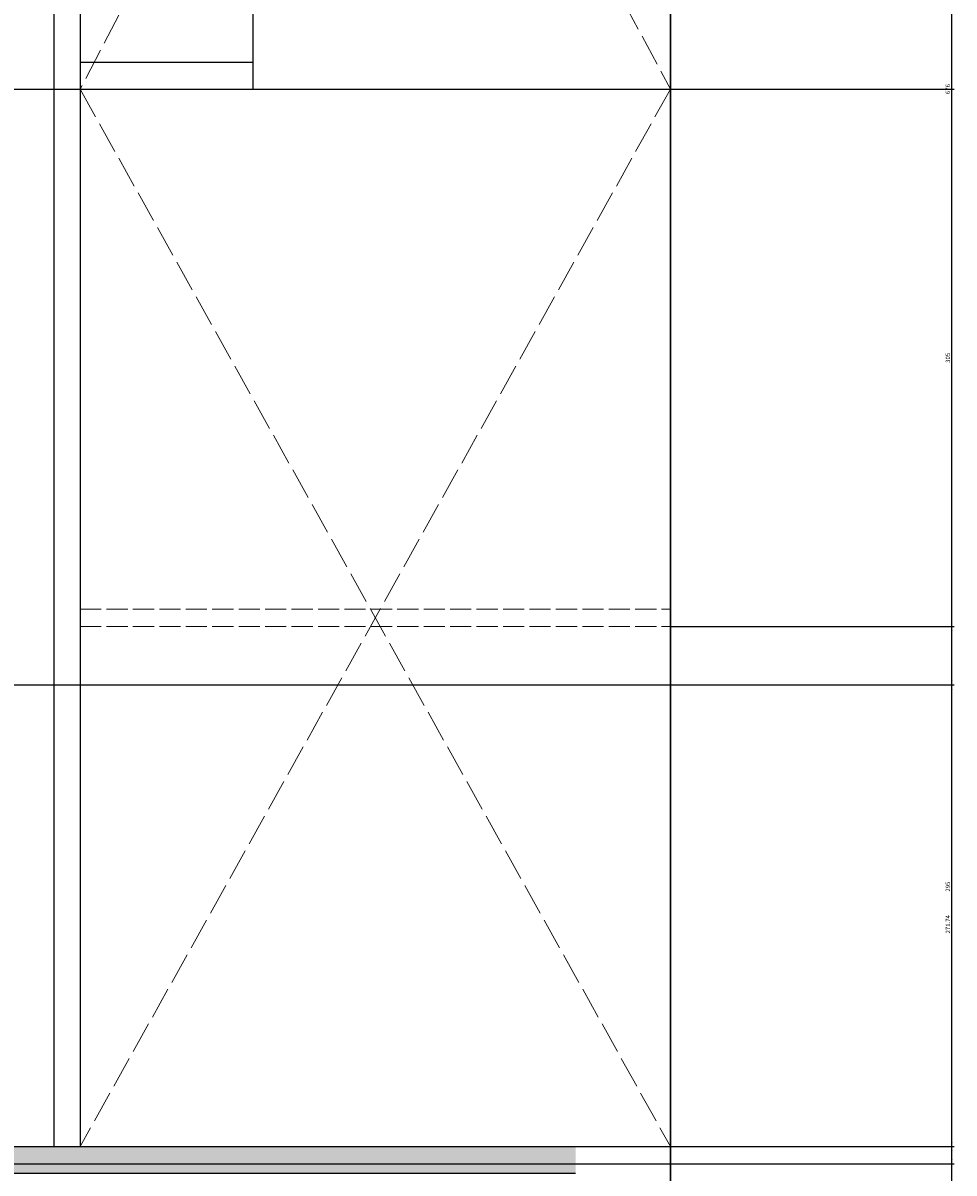
# Model space of a CAD drawing. Units: millimetres. Extents: x 2332 to 5836, y -853 to 2199.
# Tile 15 of 16: x 5308 to 5836, y 753 to 1405. Entities that reach past the tile are written whole.
import ezdxf

# ---------------------------------------------------------------- set-up
doc = ezdxf.new("R2010")
doc.units = ezdxf.units.MM
doc.linetypes.add('ACAD_ISO02W100', pattern=[15, 12, -3])
doc.layers.get('0').update_dxf_attribs({"color": 8})
for name, color, linetype, lineweight in [('A-ANNO-DIMS', 2, 'Continuous', 18), ('A-CSWK-HIDN', 8, 'ACAD_ISO02W100', 13), ('A-CSWK-PATT', 40, 'Continuous', 13), ('A-WALL', 8, 'Continuous', 30), ('SHELF', 40, 'Continuous', 25)]:
    doc.layers.add(name, color=color, linetype=linetype, lineweight=lineweight)
doc.styles.get("Standard").update_dxf_attribs({"font": 'arial.ttf'})
doc.dimstyles.new('ISO-25', dxfattribs={"dimtxt": 2.5, "dimasz": 2.5, "dimexe": 1.25, "dimexo": 0.625, "dimtad": 1, "dimtxsty": 'Standard', "dimcen": 2.5, "dimadec": 0, "dimazin": 0, "dimtfac": 1, "dimtmove": 0, "dimatfit": 3, "dimfxl": 1, "dimarcsym": 0})

# ---------------------------------------------------------------- blocks, each defined once
blk = doc.blocks.new('CAB-END-STILE')
for p, q in [((0, 1240), (0, 600)), ((98.09, 1240), (98.09, 0)), ((113.09, 1240), (113.09, 0)), ((0, 615), (98.09, 615))]:
    blk.add_line(p, q)
blk = doc.blocks.new('*D18')
at = {"layer": 'A-ANNO-DIMS', "color": 0, "lineweight": -2, "transparency": 16777216}
for p, q in [((5675.66, 767.8), (5835.94, 767.8)), ((5834.69, -689.7), (5834.69, 765.3)), ((5675.66, -692.2), (5835.94, -692.2))]:
    blk.add_line(p, q, dxfattribs=at)
at = {"layer": 'A-ANNO-DIMS', "color": 0, "transparency": 16777216}
for points in [[(5834.27, 765.3), (5835.11, 765.3), (5834.69, 767.8)], [(5834.27, -689.7), (5835.11, -689.7), (5834.69, -692.2)]]:
    blk.add_solid(points, dxfattribs=at)
at = {"layer": 'Defpoints', "color": 0, "transparency": 16777216}
for p in [(5675.04, 767.8), (5834.69, 767.8), (5675.04, -692.2)]:
    blk.add_point(p, dxfattribs=at)
at = {"layer": 'A-ANNO-DIMS', "color": 0, "transparency": 16777216, "insert": (5832.79, 37.8), "char_height": 2.5, "attachment_point": 5, "rotation": 90}
blk.add_mtext('1460', dxfattribs=at)
blk = doc.blocks.new('*D19')
at = {"layer": 'A-ANNO-DIMS', "color": 0, "lineweight": -2, "transparency": 16777216}
for p, q in [((5675.66, 1062.8), (5835.94, 1062.8)), ((5834.69, 770.3), (5834.69, 1060.3)), ((5675.66, 767.8), (5835.94, 767.8))]:
    blk.add_line(p, q, dxfattribs=at)
at = {"layer": 'A-ANNO-DIMS', "color": 0, "transparency": 16777216}
for points in [[(5834.27, 1060.3), (5835.11, 1060.3), (5834.69, 1062.8)], [(5834.27, 770.3), (5835.11, 770.3), (5834.69, 767.8)]]:
    blk.add_solid(points, dxfattribs=at)
at = {"layer": 'Defpoints', "color": 0, "transparency": 16777216}
for p in [(5675.04, 1062.8), (5834.69, 1062.8), (5675.04, 767.8)]:
    blk.add_point(p, dxfattribs=at)
at = {"layer": 'A-ANNO-DIMS', "color": 0, "transparency": 16777216, "insert": (5832.79, 915.3), "char_height": 2.5, "attachment_point": 5, "rotation": 90}
blk.add_mtext('295', dxfattribs=at)
blk = doc.blocks.new('*D20')
at = {"layer": 'A-ANNO-DIMS', "color": 0, "lineweight": -2, "transparency": 16777216}
for p, q in [((5675.66, 1367.8), (5835.94, 1367.8)), ((5834.69, 1065.3), (5834.69, 1365.3)), ((5675.66, 1062.8), (5835.94, 1062.8))]:
    blk.add_line(p, q, dxfattribs=at)
at = {"layer": 'A-ANNO-DIMS', "color": 0, "transparency": 16777216}
for points in [[(5834.27, 1365.3), (5835.11, 1365.3), (5834.69, 1367.8)], [(5834.27, 1065.3), (5835.11, 1065.3), (5834.69, 1062.8)]]:
    blk.add_solid(points, dxfattribs=at)
at = {"layer": 'Defpoints', "color": 0, "transparency": 16777216}
for p in [(5675.04, 1367.8), (5834.69, 1367.8), (5675.04, 1062.8)]:
    blk.add_point(p, dxfattribs=at)
at = {"layer": 'A-ANNO-DIMS', "color": 0, "transparency": 16777216, "insert": (5832.79, 1215.3), "char_height": 2.5, "attachment_point": 5, "rotation": 90}
blk.add_mtext('305', dxfattribs=at)
blk = doc.blocks.new('*D25')
at = {"layer": 'A-ANNO-DIMS', "color": 0, "lineweight": -2, "transparency": 16777216}
for p, q in [((4341.52, 1705.81), (5835.94, 1705.81)), ((5834.69, 1032.3), (5834.69, 1703.31)), ((4341.52, 1029.8), (5835.94, 1029.8))]:
    blk.add_line(p, q, dxfattribs=at)
at = {"layer": 'A-ANNO-DIMS', "color": 0, "transparency": 16777216}
for points in [[(5834.27, 1703.31), (5835.11, 1703.31), (5834.69, 1705.81)], [(5834.27, 1032.3), (5835.11, 1032.3), (5834.69, 1029.8)]]:
    blk.add_solid(points, dxfattribs=at)
at = {"layer": 'Defpoints', "color": 0, "transparency": 16777216}
for p in [(4340.89, 1705.81), (5834.69, 1705.81), (4340.89, 1029.8)]:
    blk.add_point(p, dxfattribs=at)
at = {"layer": 'A-ANNO-DIMS', "color": 0, "transparency": 16777216, "insert": (5832.79, 1367.8), "char_height": 2.5, "attachment_point": 5, "rotation": 90}
blk.add_mtext('676', dxfattribs=at)
blk = doc.blocks.new('*D26')
at = {"layer": 'A-ANNO-DIMS', "color": 0, "lineweight": -2, "transparency": 16777216}
for p, q in [((4774.24, 1029.8), (5835.94, 1029.8)), ((5834.69, 760.56), (5834.69, 1027.3)), ((4741.16, 758.06), (5835.94, 758.06))]:
    blk.add_line(p, q, dxfattribs=at)
at = {"layer": 'A-ANNO-DIMS', "color": 0, "transparency": 16777216}
for points in [[(5834.27, 1027.3), (5835.11, 1027.3), (5834.69, 1029.8)], [(5834.27, 760.56), (5835.11, 760.56), (5834.69, 758.06)]]:
    blk.add_solid(points, dxfattribs=at)
at = {"layer": 'Defpoints', "color": 0, "transparency": 16777216}
for p in [(4773.61, 1029.8), (5834.69, 1029.8), (4740.54, 758.06)]:
    blk.add_point(p, dxfattribs=at)
at = {"layer": 'A-ANNO-DIMS', "color": 0, "transparency": 16777216, "insert": (5832.81, 893.93), "char_height": 2.5, "attachment_point": 5, "rotation": 90}
blk.add_mtext('271.74', dxfattribs=at)

msp = doc.modelspace()

# ---------------------------------------------------------------- hatches: boundary and pattern name
at = {"layer": 'A-CSWK-PATT'}
h = msp.add_hatch(color=256, dxfattribs=at)
h.dxf.hatch_style = 1
h.paths.add_polyline_path([(4785.04, 767.803), (5285.04, 767.803), (5325.04, 767.803), (5621.17, 767.803), (5621.17, 752.803), (4785.04, 752.803)])

# ---------------------------------------------------------------- linework, layer by layer
at = {"layer": 'A-CSWK-HIDN', "ltscale": 1.5}
for p, q in [((5675.04, 2007.803), (5340.04, 1367.803)), ((5340.04, 1992.803), (5675.04, 1367.803)), ((5675.04, 1367.803), (5340.04, 767.803)), ((5340.04, 1367.803), (5675.04, 767.803))]:
    msp.add_line(p, q, dxfattribs=at)
at = {"layer": 'A-CSWK-HIDN'}
for p, q in [((5340.04, 1072.803), (5675.04, 1072.803)), ((5340.04, 1062.803), (5675.04, 1062.803))]:
    msp.add_line(p, q, dxfattribs=at)
at = {"layer": 'A-WALL'}
for p, q in [((5675.04, 1967.803), (5675.04, 1367.803)), ((5675.04, 1367.803), (5675.04, 767.803)), ((5675.04, 767.803), (5675.04, 167.803))]:
    msp.add_line(p, q, dxfattribs=at)
at = {"layer": 'SHELF'}
for p, q in [((4785.04, 1367.803), (5675.04, 1367.803)), ((5285.04, 767.803), (5325.04, 767.803)), ((5325.04, 767.803), (5675.04, 767.803)), ((4785.04, 752.803), (5621.17, 752.803))]:
    msp.add_line(p, q, dxfattribs=at)

# ---------------------------------------------------------------- block references
at = {"layer": 'SHELF', "extrusion": (0, 0, -1), "zscale": -1}
msp.add_blockref('CAB-END-STILE', (-5438.13, 767.803), dxfattribs=at)

# ---------------------------------------------------------------- dimensions: what is measured, and where the dimension line sits
at = {"layer": 'A-ANNO-DIMS'}
for base, p1, p2, override, picture, middle in [((5834.69, 1705.805), (4340.894, 1029.801), (4340.894, 1705.805), {"dimdec": 0, "dimlfac": 1, "dimrnd": 0, "dimzin": 0, "dimdsep": 46, "dimlunit": 2}, '*D25', (5832.788, 1367.803)), ((5834.69, 1367.803), (5675.04, 1062.803), (5675.04, 1367.803), {"dimdec": 0, "dimlfac": 1, "dimrnd": 0, "dimzin": 0, "dimdsep": 46, "dimlunit": 2}, '*D20', (5832.788, 1215.303)), ((5834.69, 1062.803), (5675.04, 767.803), (5675.04, 1062.803), {"dimdec": 0, "dimlfac": 1, "dimrnd": 0, "dimzin": 0, "dimdsep": 46, "dimlunit": 2}, '*D19', (5832.788, 915.303)), ((5834.69, 1029.801), (4740.539, 758.058), (4773.612, 1029.801), {"dimdec": 2, "dimlfac": 1, "dimrnd": 0, "dimzin": 0, "dimdsep": 46, "dimlunit": 2}, '*D26', (5832.81, 893.93)), ((5834.69, 767.803), (5675.04, -692.197), (5675.04, 767.803), {"dimdec": 0, "dimlfac": 1, "dimrnd": 0, "dimzin": 0, "dimdsep": 46, "dimlunit": 2}, '*D18', (5832.788, 37.803))]:
    dim = msp.add_linear_dim(base=base, p1=p1, p2=p2, angle=90, dimstyle='ISO-25', override=override, dxfattribs=at)
    dim.commit()
    dim.dimension.update_dxf_attribs({"geometry": picture, "text_midpoint": middle})

doc.saveas('drawing.dxf')
